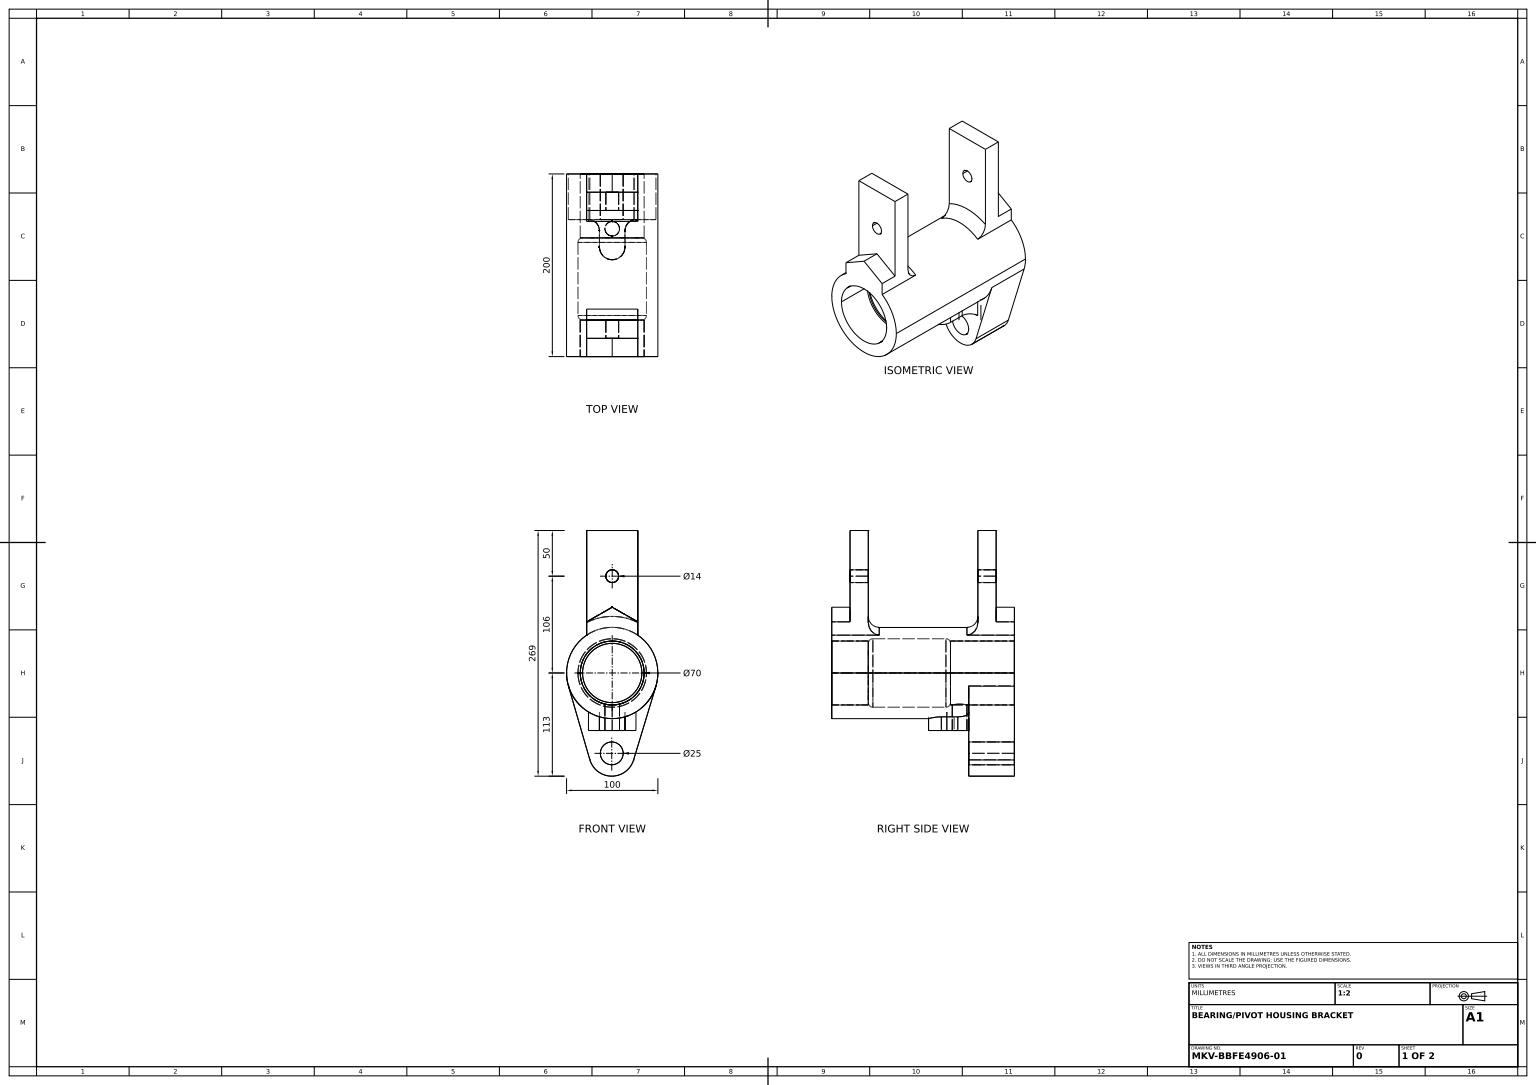
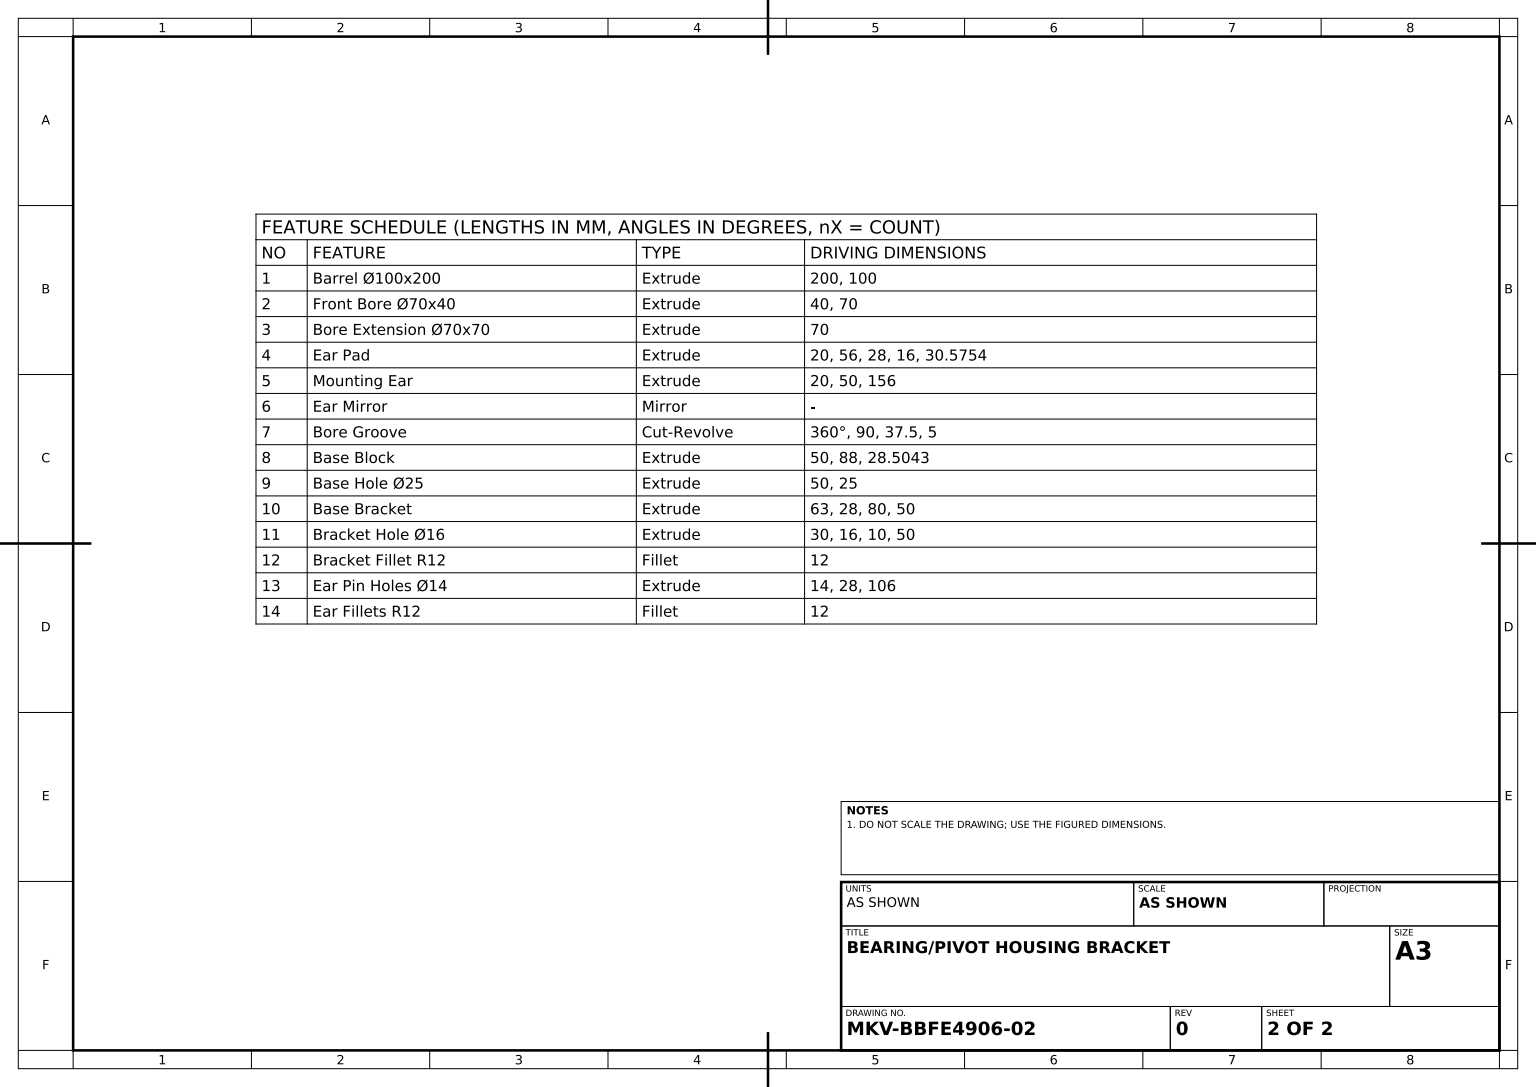
SolidWorks part; units mm, degrees
material "Plain Carbon Steel"
ref_plane "Front Plane" through (0, 0, 0) normal (0, 0, 1) x (1, 0, 0)
ref_plane "Top Plane" through (0, 0, 0) normal (0, 1, 0) x (1, 0, 0)
ref_plane "Right Plane" through (0, 0, 0) normal (1, 0, 0) x (0, 0, -1)
sketch "Barrel Profile Ø100" plane through (0, 0, 0) normal (0, 0, 1) x (1, 0, 0)
  circle A0 centre (0, 0) radius 50
  dimension "D1" = 100
extrude "Barrel Ø100x200" add sketch "Barrel Profile Ø100" against normal blind 200
sketch "Front Bore Profile Ø70" plane through (0, 0, 0) normal (0, 0, 1) x (1, 0, 0)
  circle A0 centre (0, 0) radius 35
  dimension "D1" = 70
extrude "Front Bore Ø70x40" cut sketch "Front Bore Profile Ø70" against normal blind 40
sketch "Bore Extension Profile" plane through (0, 0, -200) normal (0, 0, -1) x (-1, 0, 0)
  circle A0 centre (0, 0) radius 35 construction
  circle A1 centre (0, 0) radius 35
extrude "Bore Extension Ø70x70" cut sketch "Bore Extension Profile" against normal blind 70
ref_plane "Ear Pad Plane" through (0, 0, 0) normal (0, 0, 1) x (1, 0, 0)
sketch "Ear Pad Profile" plane through (0, 0, 0) normal (0, 0, 1) x (1, 0, 0)
  line L2 (-28, 41.4246) -> (-28, 56)
  line L4 (28, 41.4246) -> (28, 56)
  line L5 (-28, 56) -> (0, 72)
  line L6 (28, 56) -> (0, 72)
  circle A0 centre (0, 0) radius 50 construction
  arc A1 (28, 41.4246) -> (-28, 41.4246) centre (0, 0) ccw
  dimension "D1" = 16
  dimension "D2" = 56
  dimension "D3" = 28
  dimension "D4" = 56
  dimension "D5" = 28
  dimension "D6" = 30.5754
extrude "Ear Pad" add sketch "Ear Pad Profile" against normal blind 20
sketch "Ear Profile" plane through (0, 0, -20) normal (0, 0, -1) x (-1, 0, 0)
  line L0 (-28, 41.4246) -> (-28, 56)
  line L1 (-28, 56) -> (-28, 156)
  line L2 (-28, 156) -> (28, 156)
  line L3 (28, 156) -> (28, 41.4246)
  arc A0 (-28, 41.4246) -> (28, 41.4246) centre (0, 0) cw
  dimension "D1" = 50
  dimension "D2" = 156
extrude "Mounting Ear" add sketch "Ear Profile" along normal blind 20
ref_plane "Plane2" through (0, 0, -100) normal (0, 0, 1) x (1, 0, 0)
ref_plane "Ear Mirror Plane" through (0, 0, -100) normal (0, 0, 1) x (1, 0, 0)
mirror "Ear Mirror" about plane through (0, 0, -100) normal (0, 0, 1) of "Mounting Ear", "Ear Pad"
ref_plane "Groove Section Plane" through (0, 0, 0) normal (1, 0, 0) x (0, 0, -1)
sketch "Bore Groove Profile" plane through (0, 0, 0) normal (1, 0, 0) x (0, 0, -1)
  line L0 (40, 0) -> (130, 0) construction
  line L1 (40, 35) -> (40, -35) construction
  line L2 (40, 0) -> (40, 32.5)
  line L3 (45, 37.5) -> (125, 37.5)
  line L4 (130, 32.5) -> (130, 0)
  line L5 (40, 0) -> (130, 0)
  arc A0 (125, 37.5) -> (130, 32.5) centre (125, 32.5) cw
  arc A1 (40, 32.5) -> (45, 37.5) centre (45, 32.5) cw
  point P9 (130, 37.5)
  point P12 (40, 37.5)
  dimension "D3" = 5
  dimension "D1" = 90
  dimension "D2" = 37.5
revolve "Bore Groove" cut sketch "Bore Groove Profile" angle 360 about L0
sketch "Base Block Profile" plane through (0, 0, -200) normal (0, 0, -1) x (-1, 0, 0)
  line L0 (-23.4245, -95.2381) -> (-47.8577, -14.479)
  line L1 (24.5145, -94.9633) -> (48.0205, -13.9296)
  arc A0 (-23.4245, -95.2381) -> (24.5145, -94.9633) centre (0.5043, -87.9986) ccw
  arc A2 (-28, 41.4246) -> (28, 41.4246) centre (0, 0) ccw construction
  arc A3 (-47.8577, -14.479) -> (48.0205, -13.9296) centre (0, 0) ccw
  dimension "D1" = 50
  dimension "D3" = 28.5043
  dimension "D2" = 88
extrude "Base Block" add sketch "Base Block Profile" against normal blind 50
sketch "Base Hole Profile Ø25" plane through (0, 0, -150) normal (0, 0, 1) x (1, 0, 0)
  circle A0 centre (-0.5043, -87.9986) radius 12.5
  dimension "D1" = 25
extrude "Base Hole Ø25" cut sketch "Base Hole Profile Ø25" against normal blind 50
ref_plane "Bracket Plane" through (0, -63, 0) normal (0, 1, 0) x (1, 0, 0)
sketch "Base Bracket Profile" plane through (0, -63, 0) normal (0, 1, 0) x (1, 0, 0)
  line L0 (23.4245, 200) -> (-24.5145, 200) construction
  line L1 (-50, 200) -> (-50, 0) construction
  line L2 (-14, 120) -> (-14, 150)
  line L3 (-48.0205, 150) -> (47.8577, 150) construction
  line L4 (-14, 150) -> (14, 150)
  line L5 (14, 150) -> (14, 120)
  arc A0 (-14, 120) -> (14, 120) centre (0, 120) ccw
  dimension "D1" = 28
  dimension "D2" = 80
  dimension "D3" = 50
extrude "Base Bracket" add sketch "Base Bracket Profile" along normal up to next
sketch "Bracket Hole Profile Ø16" plane through (0, -63, 0) normal (0, -1, 0) x (1, 0, 0)
  line L0 (23.4245, -150) -> (-24.5145, -150) construction
  line L1 (-50, 0) -> (-50, -200) construction
  circle A0 centre (0, -140) radius 8
  dimension "D1" = 16
  dimension "D2" = 10
  dimension "D3" = 50
extrude "Bracket Hole Ø16" cut sketch "Bracket Hole Profile Ø16" against normal blind 30
fillet "Bracket Fillet R12" radius 12 2 edges at (-14, -55.5, -150) (14, -55.5, -150)
sketch "Ear Pin Hole Profile Ø14" plane through (0, 0, -20) normal (0, 0, 1) x (1, 0, 0)
  line L0 (-28, 56) -> (-28, 156) construction
  circle A0 centre (0, 106) radius 7
  dimension "D1" = 14
  dimension "D2" = 28
  dimension "D3" = 106
extrude "Ear Pin Holes Ø14" cut sketch "Ear Pin Hole Profile Ø14" against normal through all
fillet "Ear Fillets R12" radius 12 2 edges at (0, 50, -40) (0, 50, -160)
